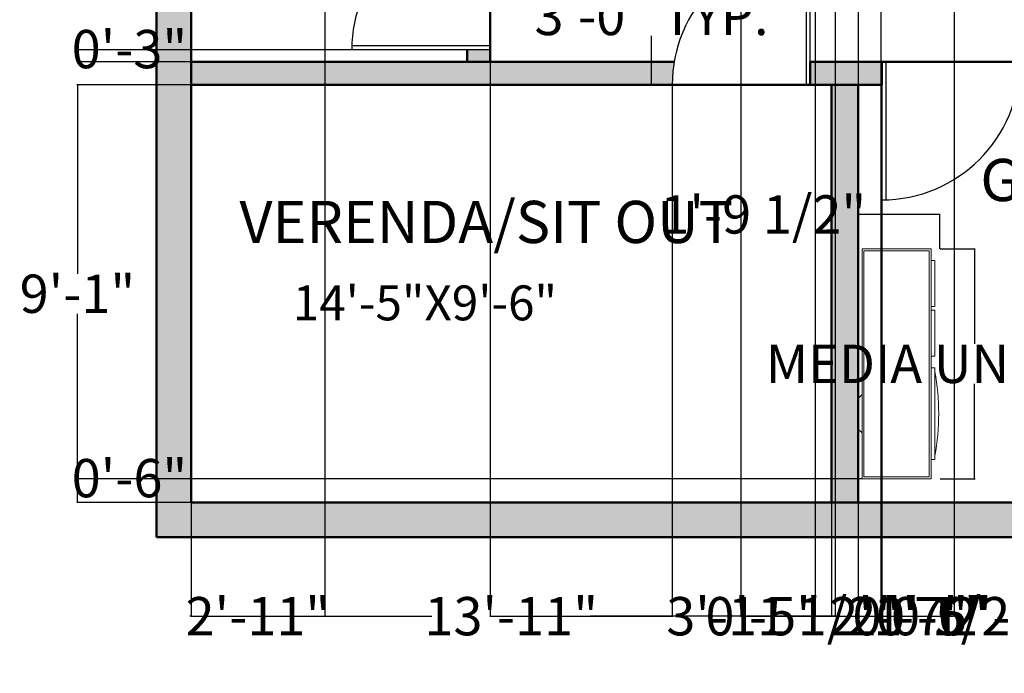
# Model space of a CAD drawing. Units: inches. Extents: x 168 to 640, y -211 to 244.
# Tile 1 of 3: x 179 to 436, y -211 to -40. Entities that reach past the tile are written whole.
import ezdxf

# ---------------------------------------------------------------- set-up
doc = ezdxf.new("R2010")
doc.units = ezdxf.units.IN
doc.header["$MEASUREMENT"] = 0
for name, color, linetype, lineweight in [('A-ANNO-DIMS', 2, 'Continuous', 18), ('A-AREA-IDEN', 7, 'Continuous', 25), ('A-DOOR', 4, 'Continuous', 25), ('A-FURN', 8, 'Continuous', 18), ('A-WALL', 7, 'Continuous', 50)]:
    doc.layers.add(name, color=color, linetype=linetype, lineweight=lineweight)
doc.layers.add('A-WALL-PATT', color=251, linetype='Continuous', lineweight=13, true_color=0x636466)
doc.styles.get("Standard").update_dxf_attribs({"font": 'arial.ttf'})
doc.dimstyles.get("Standard").update_dxf_attribs({"dimtxt": 10, "dimasz": 0.18, "dimexe": 0.18, "dimexo": 0.0625, "dimgap": 0.09, "dimtad": 0, "dimtih": 1, "dimtoh": 1, "dimdec": 0, "dimzin": 0, "dimdsep": 46, "dimlunit": 3, "dimtxsty": 'Standard', "dimcen": 0.09, "dimadec": 0, "dimazin": 0, "dimtfac": 1, "dimtdec": 0, "dimtofl": 0, "dimtmove": 0, "dimatfit": 3, "dimfxl": 1, "dimtolj": 1, "dimtzin": 0, "dimarcsym": 0})

# ---------------------------------------------------------------- blocks, each defined once
blk = doc.blocks.new('Entertainment Center')
for p, q in [((-4, 0), (-5, -1)), ((4, 0), (-4, 0)), ((5, -1), (4, 0)), ((-17, -19), (-17, -1)), ((-17, -1), (43, -1)), ((-16.5, -18.5), (-16.5, -1.5)), ((-16.5, -1.5), (42.5, -1.5)), ((42.5, -1.5), (42.5, -18.5)), ((43, -1), (43, -19)), ((43, -19), (-17, -19)), ((42.5, -18.5), (-16.5, -18.5)), ((-12, -20), (-12, -19)), ((12, -20), (-12, -20)), ((12, -19), (12, -20)), ((15, -20), (15, -19)), ((27, -20), (15, -20)), ((27, -19), (27, -20)), ((28, -20), (28, -19)), ((40, -20), (28, -20)), ((40, -19), (40, -20))]:
    blk.add_line(p, q)
blk.add_arc((0, 40), 61, 259.6111, 280.3889)
blk = doc.blocks.new('DOOR-SWING-36IN')
for p, q in [((0, 36), (0, 0)), ((1, 36), (1, 0))]:
    blk.add_line(p, q)
blk.add_arc((0, 36), 36, 270, 0)
blk = doc.blocks.new('*D12')
at = {"layer": 'A-ANNO-DIMS', "color": 0, "lineweight": -2, "ltscale": 0.25, "transparency": 16777216}
for p, q in [((349.06, -21.2), (343.54, -21.2)), ((343.72, -21.38), (343.72, -34)), ((343.72, -57.02), (343.72, -44.4)), ((349.06, -57.2), (343.54, -57.2))]:
    blk.add_line(p, q, dxfattribs=at)
at = {"layer": 'A-ANNO-DIMS', "color": 0, "ltscale": 0.25, "transparency": 16777216}
for points in [[(343.69, -21.38), (343.75, -21.38), (343.72, -21.2)], [(343.69, -57.02), (343.75, -57.02), (343.72, -57.2)]]:
    blk.add_solid(points, dxfattribs=at)
at = {"layer": 'Defpoints', "color": 0, "ltscale": 0.25, "transparency": 16777216}
for p in [(349.12, -21.2), (343.72, -57.2), (349.12, -57.2)]:
    blk.add_point(p, dxfattribs=at)
at = {"layer": 'A-ANNO-DIMS', "color": 0, "ltscale": 0.25, "transparency": 16777216, "insert": (343.72, -39.2), "char_height": 10, "attachment_point": 5}
blk.add_mtext('\\A1;3\'-0" TYP.', dxfattribs=at)
blk = doc.blocks.new('*D19')
at = {"layer": 'A-ANNO-DIMS', "color": 0, "lineweight": -2, "ltscale": 0.25, "transparency": 16777216}
for p, q in [((419.03, -100), (428.15, -100)), ((427.97, -100.18), (427.97, -124.81)), ((427.97, -159.82), (427.97, -135.2)), ((419.03, -160), (428.15, -160))]:
    blk.add_line(p, q, dxfattribs=at)
at = {"layer": 'A-ANNO-DIMS', "color": 0, "ltscale": 0.25, "transparency": 16777216}
for points in [[(427.94, -100.18), (428, -100.18), (427.97, -100)], [(427.94, -159.82), (428, -159.82), (427.97, -160)]]:
    blk.add_solid(points, dxfattribs=at)
at = {"layer": 'Defpoints', "color": 0, "ltscale": 0.25, "transparency": 16777216}
for p in [(418.97, -100), (427.97, -100), (418.97, -160)]:
    blk.add_point(p, dxfattribs=at)
at = {"layer": 'A-ANNO-DIMS', "color": 0, "ltscale": 0.25, "transparency": 16777216, "insert": (427.97, -130), "char_height": 10, "attachment_point": 5}
blk.add_mtext('\\A1;MEDIA UNIT 5\'-0"', dxfattribs=at)
blk = doc.blocks.new('*D20')
at = {"layer": 'A-ANNO-DIMS', "color": 0, "lineweight": -2, "ltscale": 0.25, "transparency": 16777216}
for p, q in [((397.63, -91), (397.45, -91)), ((397.63, -99.94), (397.63, -90.82)), ((418.79, -91), (397.81, -91)), ((418.97, -99.94), (418.97, -90.82))]:
    blk.add_line(p, q, dxfattribs=at)
at = {"layer": 'A-ANNO-DIMS', "color": 0, "ltscale": 0.25, "transparency": 16777216}
for points in [[(397.81, -90.97), (397.81, -91.03), (397.63, -91)], [(418.79, -90.97), (418.79, -91.03), (418.97, -91)]]:
    blk.add_solid(points, dxfattribs=at)
at = {"layer": 'Defpoints', "color": 0, "ltscale": 0.25, "transparency": 16777216}
for p in [(397.63, -91), (397.63, -100), (418.97, -100)]:
    blk.add_point(p, dxfattribs=at)
at = {"layer": 'A-ANNO-DIMS', "color": 0, "ltscale": 0.25, "transparency": 16777216, "insert": (372.89, -91), "char_height": 10, "attachment_point": 5}
blk.add_mtext('\\A1;1\'-9 1/2"', dxfattribs=at)
blk = doc.blocks.new('*D28')
at = {"layer": 'A-ANNO-DIMS', "color": 0, "lineweight": -2, "ltscale": 0.25, "transparency": 16777216}
for p, q in [((390.63, -166.26), (390.63, -196.03)), ((397.63, -166.26), (397.63, -196.03)), ((390.81, -195.85), (397.45, -195.85)), ((397.63, -195.85), (397.81, -195.85))]:
    blk.add_line(p, q, dxfattribs=at)
at = {"layer": 'A-ANNO-DIMS', "color": 0, "ltscale": 0.25, "transparency": 16777216}
for points in [[(390.81, -195.82), (390.81, -195.88), (390.63, -195.85)], [(397.45, -195.82), (397.45, -195.88), (397.63, -195.85)]]:
    blk.add_solid(points, dxfattribs=at)
at = {"layer": 'Defpoints', "color": 0, "ltscale": 0.25, "transparency": 16777216}
for p in [(390.63, -166.2), (397.63, -166.2), (397.63, -195.85)]:
    blk.add_point(p, dxfattribs=at)
at = {"layer": 'A-ANNO-DIMS', "color": 0, "ltscale": 0.25, "transparency": 16777216, "insert": (411.2, -195.85), "char_height": 10, "attachment_point": 5}
blk.add_mtext('\\A1;0\'-7"', dxfattribs=at)
blk = doc.blocks.new('*D29')
at = {"layer": 'A-ANNO-DIMS', "color": 0, "lineweight": -2, "ltscale": 0.25, "transparency": 16777216}
for p, q in [((223.63, -166.26), (223.63, -196.03)), ((390.63, -166.26), (390.63, -196.03)), ((223.81, -195.85), (286.45, -195.85)), ((390.45, -195.85), (327.81, -195.85))]:
    blk.add_line(p, q, dxfattribs=at)
at = {"layer": 'A-ANNO-DIMS', "color": 0, "ltscale": 0.25, "transparency": 16777216}
for points in [[(223.81, -195.82), (223.81, -195.88), (223.63, -195.85)], [(390.45, -195.82), (390.45, -195.88), (390.63, -195.85)]]:
    blk.add_solid(points, dxfattribs=at)
at = {"layer": 'Defpoints', "color": 0, "ltscale": 0.25, "transparency": 16777216}
for p in [(223.63, -166.2), (390.63, -166.2), (390.63, -195.85)]:
    blk.add_point(p, dxfattribs=at)
at = {"layer": 'A-ANNO-DIMS', "color": 0, "ltscale": 0.25, "transparency": 16777216, "insert": (307.13, -195.85), "char_height": 10, "attachment_point": 5}
blk.add_mtext('\\A1;13\'-11"', dxfattribs=at)
blk = doc.blocks.new('*D30')
at = {"layer": 'A-ANNO-DIMS', "color": 0, "lineweight": -2, "ltscale": 0.25, "transparency": 16777216}
for p, q in [((223.57, -57.2), (193.8, -57.2)), ((193.98, -57.38), (193.98, -106.5)), ((193.98, -166.02), (193.98, -116.9)), ((223.57, -166.2), (193.8, -166.2))]:
    blk.add_line(p, q, dxfattribs=at)
at = {"layer": 'A-ANNO-DIMS', "color": 0, "ltscale": 0.25, "transparency": 16777216}
for points in [[(193.95, -57.38), (194.01, -57.38), (193.98, -57.2)], [(193.95, -166.02), (194.01, -166.02), (193.98, -166.2)]]:
    blk.add_solid(points, dxfattribs=at)
at = {"layer": 'Defpoints', "color": 0, "ltscale": 0.25, "transparency": 16777216}
for p in [(193.98, -57.2), (223.63, -57.2), (223.63, -166.2)]:
    blk.add_point(p, dxfattribs=at)
at = {"layer": 'A-ANNO-DIMS', "color": 0, "ltscale": 0.25, "transparency": 16777216, "insert": (193.98, -111.7), "char_height": 10, "attachment_point": 5}
blk.add_mtext('\\A1;9\'-1"', dxfattribs=at)
blk = doc.blocks.new('*D35')
at = {"layer": 'A-ANNO-DIMS', "color": 0, "lineweight": -2, "ltscale": 0.25, "transparency": 16777216}
for p, q in [((386.42, 73.74), (386.42, -196.03)), ((403.56, 73.74), (403.56, -196.03)), ((386.6, -195.85), (403.38, -195.85)), ((403.56, -195.85), (403.74, -195.85))]:
    blk.add_line(p, q, dxfattribs=at)
at = {"layer": 'A-ANNO-DIMS', "color": 0, "ltscale": 0.25, "transparency": 16777216}
for points in [[(386.6, -195.82), (386.6, -195.88), (386.42, -195.85)], [(403.38, -195.82), (403.38, -195.88), (403.56, -195.85)]]:
    blk.add_solid(points, dxfattribs=at)
at = {"layer": 'Defpoints', "color": 0, "ltscale": 0.25, "transparency": 16777216}
for p in [(386.42, 73.8), (403.56, 73.8), (403.56, -195.85)]:
    blk.add_point(p, dxfattribs=at)
at = {"layer": 'A-ANNO-DIMS', "color": 0, "ltscale": 0.25, "transparency": 16777216, "insert": (416.65, -195.85), "char_height": 10, "attachment_point": 5}
blk.add_mtext('\\A1;1\'-5"', dxfattribs=at)
blk = doc.blocks.new('*D36')
at = {"layer": 'A-ANNO-DIMS', "color": 0, "lineweight": -2, "ltscale": 0.25, "transparency": 16777216}
for p, q in [((386.42, 79.74), (386.42, -196.03)), ((391.63, 79.74), (391.63, -196.03)), ((386.42, -195.85), (386.24, -195.85)), ((391.45, -195.85), (386.6, -195.85))]:
    blk.add_line(p, q, dxfattribs=at)
at = {"layer": 'A-ANNO-DIMS', "color": 0, "ltscale": 0.25, "transparency": 16777216}
for points in [[(386.6, -195.82), (386.6, -195.88), (386.42, -195.85)], [(391.45, -195.82), (391.45, -195.88), (391.63, -195.85)]]:
    blk.add_solid(points, dxfattribs=at)
at = {"layer": 'Defpoints', "color": 0, "ltscale": 0.25, "transparency": 16777216}
for p in [(386.42, 79.8), (391.63, 79.8), (386.42, -195.85)]:
    blk.add_point(p, dxfattribs=at)
at = {"layer": 'A-ANNO-DIMS', "color": 0, "ltscale": 0.25, "transparency": 16777216, "insert": (372.86, -195.85), "char_height": 10, "attachment_point": 5}
blk.add_mtext('\\A1;0\'-5"', dxfattribs=at)
blk = doc.blocks.new('*D37')
at = {"layer": 'A-ANNO-DIMS', "color": 0, "lineweight": -2, "ltscale": 0.25, "transparency": 16777216}
for p, q in [((301.63, -51.26), (301.63, -196.03)), ((349.12, -57.26), (349.12, -196.03)), ((301.81, -195.85), (348.94, -195.85)), ((349.12, -195.85), (349.3, -195.85))]:
    blk.add_line(p, q, dxfattribs=at)
at = {"layer": 'A-ANNO-DIMS', "color": 0, "ltscale": 0.25, "transparency": 16777216}
for points in [[(301.81, -195.82), (301.81, -195.88), (301.63, -195.85)], [(348.94, -195.82), (348.94, -195.88), (349.12, -195.85)]]:
    blk.add_solid(points, dxfattribs=at)
at = {"layer": 'Defpoints', "color": 0, "ltscale": 0.25, "transparency": 16777216}
for p in [(301.63, -51.2), (349.12, -57.2), (349.12, -195.85)]:
    blk.add_point(p, dxfattribs=at)
at = {"layer": 'A-ANNO-DIMS', "color": 0, "ltscale": 0.25, "transparency": 16777216, "insert": (378.21, -195.85), "char_height": 10, "attachment_point": 5}
blk.add_mtext('\\A1;3\'-11 1/2"', dxfattribs=at)
blk = doc.blocks.new('*D38')
at = {"layer": 'A-ANNO-DIMS', "color": 0, "lineweight": -2, "ltscale": 0.25, "transparency": 16777216}
for p, q in [((397.63, -57.26), (397.63, -196.03)), ((403.8, -57.26), (403.8, -196.03)), ((397.81, -195.85), (403.62, -195.85)), ((403.8, -195.85), (403.98, -195.85))]:
    blk.add_line(p, q, dxfattribs=at)
at = {"layer": 'A-ANNO-DIMS', "color": 0, "ltscale": 0.25, "transparency": 16777216}
for points in [[(397.81, -195.82), (397.81, -195.88), (397.63, -195.85)], [(403.62, -195.82), (403.62, -195.88), (403.8, -195.85)]]:
    blk.add_solid(points, dxfattribs=at)
at = {"layer": 'Defpoints', "color": 0, "ltscale": 0.25, "transparency": 16777216}
for p in [(397.63, -57.2), (403.8, -57.2), (403.8, -195.85)]:
    blk.add_point(p, dxfattribs=at)
at = {"layer": 'A-ANNO-DIMS', "color": 0, "ltscale": 0.25, "transparency": 16777216, "insert": (417.37, -195.85), "char_height": 10, "attachment_point": 5}
blk.add_mtext('\\A1;0\'-6"', dxfattribs=at)
blk = doc.blocks.new('*D39')
at = {"layer": 'A-ANNO-DIMS', "color": 0, "lineweight": -2, "ltscale": 0.25, "transparency": 16777216}
for p, q in [((295.57, -48.03), (193.8, -48.03)), ((193.98, -48.03), (193.98, -47.85)), ((193.98, -47.85), (194.16, -47.85)), ((193.98, -51.02), (193.98, -48.21)), ((295.57, -51.2), (193.8, -51.2))]:
    blk.add_line(p, q, dxfattribs=at)
at = {"layer": 'A-ANNO-DIMS', "color": 0, "ltscale": 0.25, "transparency": 16777216}
for points in [[(193.95, -48.21), (194.01, -48.21), (193.98, -48.03)], [(193.95, -51.02), (194.01, -51.02), (193.98, -51.2)]]:
    blk.add_solid(points, dxfattribs=at)
at = {"layer": 'Defpoints', "color": 0, "ltscale": 0.25, "transparency": 16777216}
for p in [(193.98, -48.03), (295.63, -48.03), (295.63, -51.2)]:
    blk.add_point(p, dxfattribs=at)
at = {"layer": 'A-ANNO-DIMS', "color": 0, "ltscale": 0.25, "transparency": 16777216, "insert": (207.55, -47.85), "char_height": 10, "attachment_point": 5}
blk.add_mtext('\\A1;0\'-3"', dxfattribs=at)
blk = doc.blocks.new('*D45')
at = {"layer": 'A-ANNO-DIMS', "color": 0, "lineweight": -2, "ltscale": 0.25, "transparency": 16777216}
for p, q in [((223.63, -20.98), (223.63, -196.03)), ((258.47, -20.98), (258.47, -196.03)), ((223.45, -195.85), (223.27, -195.85)), ((258.65, -195.85), (258.83, -195.85))]:
    blk.add_line(p, q, dxfattribs=at)
at = {"layer": 'A-ANNO-DIMS', "color": 0, "ltscale": 0.25, "transparency": 16777216}
for points in [[(223.45, -195.82), (223.45, -195.88), (223.63, -195.85)], [(258.65, -195.82), (258.65, -195.88), (258.47, -195.85)]]:
    blk.add_solid(points, dxfattribs=at)
at = {"layer": 'Defpoints', "color": 0, "ltscale": 0.25, "transparency": 16777216}
for p in [(223.63, -20.92), (258.47, -20.92), (258.47, -195.85)]:
    blk.add_point(p, dxfattribs=at)
at = {"layer": 'A-ANNO-DIMS', "color": 0, "ltscale": 0.25, "transparency": 16777216, "insert": (241.05, -195.85), "char_height": 10, "attachment_point": 5}
blk.add_mtext('\\A1;2\'-11"', dxfattribs=at)
blk = doc.blocks.new('*D53')
at = {"layer": 'A-ANNO-DIMS', "color": 0, "lineweight": -2, "ltscale": 0.25, "transparency": 16777216}
for p, q in [((367.04, 124.86), (367.04, -196.03)), ((391.63, 124.86), (391.63, -196.03)), ((367.22, -195.85), (391.45, -195.85)), ((391.63, -195.85), (391.81, -195.85))]:
    blk.add_line(p, q, dxfattribs=at)
at = {"layer": 'A-ANNO-DIMS', "color": 0, "ltscale": 0.25, "transparency": 16777216}
for points in [[(367.22, -195.82), (367.22, -195.88), (367.04, -195.85)], [(391.45, -195.82), (391.45, -195.88), (391.63, -195.85)]]:
    blk.add_solid(points, dxfattribs=at)
at = {"layer": 'Defpoints', "color": 0, "ltscale": 0.25, "transparency": 16777216}
for p in [(367.04, 124.92), (391.63, 124.92), (391.63, -195.85)]:
    blk.add_point(p, dxfattribs=at)
at = {"layer": 'A-ANNO-DIMS', "color": 0, "ltscale": 0.25, "transparency": 16777216, "insert": (416.93, -195.85), "char_height": 10, "attachment_point": 5}
blk.add_mtext('\\A1;2\'-0 1/2"', dxfattribs=at)
blk = doc.blocks.new('*D55')
at = {"layer": 'A-ANNO-DIMS', "color": 0, "lineweight": -2, "ltscale": 0.25, "transparency": 16777216}
for p, q in [((397.63, 124.86), (397.63, -196.03)), ((422.63, 124.86), (422.63, -196.03)), ((397.81, -195.85), (422.45, -195.85)), ((422.63, -195.85), (422.81, -195.85))]:
    blk.add_line(p, q, dxfattribs=at)
at = {"layer": 'A-ANNO-DIMS', "color": 0, "ltscale": 0.25, "transparency": 16777216}
for points in [[(397.81, -195.82), (397.81, -195.88), (397.63, -195.85)], [(422.45, -195.82), (422.45, -195.88), (422.63, -195.85)]]:
    blk.add_solid(points, dxfattribs=at)
at = {"layer": 'Defpoints', "color": 0, "ltscale": 0.25, "transparency": 16777216}
for p in [(397.63, 124.92), (422.63, 124.92), (422.63, -195.85)]:
    blk.add_point(p, dxfattribs=at)
at = {"layer": 'A-ANNO-DIMS', "color": 0, "ltscale": 0.25, "transparency": 16777216, "insert": (436.28, -195.85), "char_height": 10, "attachment_point": 5}
blk.add_mtext('\\A1;2\'-1"', dxfattribs=at)
blk = doc.blocks.new('*D59')
at = {"layer": 'A-ANNO-DIMS', "color": 0, "lineweight": -2, "ltscale": 0.25, "transparency": 16777216}
for p, q in [((398.57, -160), (193.8, -160)), ((193.98, -160), (193.98, -159.82)), ((193.98, -159.82), (194.16, -159.82)), ((193.98, -166.02), (193.98, -160.18)), ((397.57, -166.2), (193.8, -166.2))]:
    blk.add_line(p, q, dxfattribs=at)
at = {"layer": 'A-ANNO-DIMS', "color": 0, "ltscale": 0.25, "transparency": 16777216}
for points in [[(193.95, -160.18), (194.01, -160.18), (193.98, -160)], [(193.95, -166.02), (194.01, -166.02), (193.98, -166.2)]]:
    blk.add_solid(points, dxfattribs=at)
at = {"layer": 'Defpoints', "color": 0, "ltscale": 0.25, "transparency": 16777216}
for p in [(193.98, -160), (398.63, -160), (397.63, -166.2)]:
    blk.add_point(p, dxfattribs=at)
at = {"layer": 'A-ANNO-DIMS', "color": 0, "ltscale": 0.25, "transparency": 16777216, "insert": (207.55, -159.82), "char_height": 10, "attachment_point": 5}
blk.add_mtext('\\A1;0\'-6"', dxfattribs=at)

msp = doc.modelspace()

# ---------------------------------------------------------------- hatches: boundary and pattern name
at = {"layer": 'A-WALL-PATT', "ltscale": 0.25}
h = msp.add_hatch(color=256, dxfattribs=at)
h.dxf.hatch_style = 1
h.paths.add_polyline_path([(223.63, 11.3), (214.63, 11.3), (214.63, -175.2), (574.63, -175.2), (574.63, -137.43), (565.63, -137.43), (565.63, -157.06), (565.63, -166.2), (223.63, -166.2)])
h.paths.add_polyline_path([(349.62, -51.2), (301.63, -51.2), (223.63, -51.2), (223.63, -57.2), (301.63, -57.2), (349.12, -57.2, -0.041886)], flags=17)
h.paths.add_polyline_path([(301.63, -48.03), (295.63, -48.03), (295.63, -51.2), (301.63, -51.2)], flags=17)
h.paths.add_polyline_path([(403.8, -51.2), (385.12, -51.2), (385.12, -57.2), (403.8, -57.2)], flags=17)
h.paths.add_polyline_path([(397.63, -57.2), (390.63, -57.2), (390.63, -166.2), (397.63, -166.2)], flags=17)
h.paths.add_polyline_path([(301.63, 73.8), (295.63, 73.8), (295.63, -12.53, -0.041886), (301.63, -12.03)])
h.paths.add_polyline_path([(223.63, 122.57), (214.63, 122.57), (214.63, 47.3), (223.63, 47.3), (223.63, 73.8)])
h.paths.add_polyline_path([(350.92, 79.8), (223.63, 79.8), (223.63, 73.8), (350.42, 73.8, -0.041886)])
h.paths.add_polyline_path([(574.63, 208.8), (214.63, 208.8), (214.63, 158.57), (223.63, 158.57), (223.63, 199.8), (565.63, 199.8), (565.63, 158.57), (574.63, 158.57)])
h.paths.add_polyline_path([(397.63, 199.8), (391.63, 199.8), (391.63, 79.8), (386.42, 79.8), (386.42, 73.8), (391.63, 73.8), (403.56, 73.8), (403.56, 79.8), (397.63, 79.8)])
h.paths.add_polyline_path([(565.63, 79.8), (439.06, 79.8, -0.041886), (439.56, 73.8), (565.63, 73.8)])
h.paths.add_polyline_path([(574.63, 122.57), (565.63, 122.57), (565.63, 79.8), (565.63, 52.8), (574.63, 52.8)])
h.paths.add_polyline_path([(574.63, 16.8), (565.63, 16.8), (565.63, -15.33), (574.63, -15.33)])
h.paths.add_polyline_path([(574.63, -39.29), (570.13, -39.29), (565.63, -39.29), (565.63, -51.2), (565.63, -101.43), (574.63, -101.43)], flags=17)
h.paths.add_polyline_path([(565.63, -51.2), (439.8, -51.2, -0.041886), (439.3, -57.2), (565.63, -57.2)], flags=17)

# ---------------------------------------------------------------- linework, layer by layer
at = {"layer": 'A-DOOR'}
msp.add_line((301.63, -47.03), (301.63, -48.03), dxfattribs=at)
at = {"layer": 'A-WALL'}
for p, q in [((214.63, 208.8), (214.63, -175.2)), ((223.63, 199.8), (223.63, -166.2)), ((223.63, 73.8), (223.63, -51.2)), ((301.63, -51.2), (301.63, 73.8)), ((295.63, -51.2), (295.63, -48.03)), ((223.63, -51.2), (301.63, -51.2)), ((349.62, -51.2), (301.63, -51.2)), ((565.63, -51.2), (385.12, -51.2)), ((385.12, -57.2), (385.12, -51.2)), ((403.8, -57.2), (403.8, -51.2)), ((223.63, -57.2), (301.63, -57.2)), ((403.8, -57.2), (301.63, -57.2)), ((390.63, -57.2), (390.63, -166.2)), ((397.63, -57.2), (397.63, -166.2)), ((223.63, -166.2), (565.63, -166.2)), ((214.63, -175.2), (574.63, -175.2))]:
    msp.add_line(p, q, dxfattribs=at)

# ---------------------------------------------------------------- block references
at = {"layer": 'A-DOOR', "extrusion": (0, 0, -1), "zscale": -1, "rotation": 90.00000000000007}
msp.add_blockref('DOOR-SWING-36IN', (-265.63, -48.03), dxfattribs=at)
at = {"layer": 'A-DOOR', "rotation": 180}
msp.add_blockref('DOOR-SWING-36IN', (385.12, -21.2), dxfattribs=at)
at = {"layer": 'A-DOOR'}
msp.add_blockref('DOOR-SWING-36IN', (403.8, -87.2), dxfattribs=at)
at = {"layer": 'A-FURN', "ltscale": 0.25, "rotation": 90}
msp.add_blockref('Entertainment Center', (397.63, -143), dxfattribs=at)

# ---------------------------------------------------------------- texts
at = {"layer": 'A-AREA-IDEN', "ltscale": 0.25}
for s, height, p in [('GUEST/DRAWING', 11.0125, (429.5, -87.52)), ('VERENDA/SIT OUT  ', 11.0125, (236.23, -98.47)), ('14\'-5"X9\'-6"', 9.1115, (250.15, -118.64))]:
    msp.add_text(s, height=height, dxfattribs=at).set_placement(p)

# ---------------------------------------------------------------- dimensions: what is measured, and where the dimension line sits
at = {"layer": 'A-ANNO-DIMS', "ltscale": 0.25}
for base, p1, p2, picture, middle in [((391.63, -195.85), (367.04, 124.92), (391.63, 124.92), '*D53', (416.93, -195.85)), ((422.63, -195.85), (397.63, 124.92), (422.63, 124.92), '*D55', (436.28, -195.85)), ((386.42, -195.85), (391.63, 79.8), (386.42, 79.8), '*D36', (372.86, -195.85)), ((403.56, -195.85), (386.42, 73.8), (403.56, 73.8), '*D35', (416.65, -195.85)), ((258.47, -195.85), (223.63, -20.92), (258.47, -20.92), '*D45', (241.05, -195.85)), ((349.12, -195.85), (301.63, -51.2), (349.12, -57.2), '*D37', (378.21, -195.85)), ((403.8, -195.85), (397.63, -57.2), (403.8, -57.2), '*D38', (417.37, -195.85)), ((390.63, -195.85), (223.63, -166.2), (390.63, -166.2), '*D29', (307.13, -195.85)), ((397.63, -195.85), (390.63, -166.2), (397.63, -166.2), '*D28', (411.2, -195.85))]:
    dim = msp.add_linear_dim(base=base, p1=p1, p2=p2, dimstyle='Standard', override={"dimdec": 1, "dimlfac": 1, "dimrnd": 0, "dimzin": 1, "dimdsep": 46, "dimlunit": 4, "dimfrac": 2}, dxfattribs=at)
    dim.commit()
    dim.dimension.update_dxf_attribs({"geometry": picture, "text_midpoint": middle})
for base, p1, p2, angle, text, picture, middle in [((343.72, -57.2), (349.12, -21.2), (349.12, -57.2), 270, '<> TYP.', '*D12', (343.72, -39.2)), ((427.97, -100), (418.97, -160), (418.97, -100), 90, 'MEDIA UNIT <>', '*D19', (427.97, -130))]:
    dim = msp.add_linear_dim(base=base, p1=p1, p2=p2, angle=angle, text=text, dimstyle='Standard', override={"dimdec": 1, "dimlfac": 1, "dimrnd": 0, "dimzin": 1, "dimdsep": 46, "dimlunit": 4, "dimfrac": 2}, dxfattribs=at)
    dim.commit()
    dim.dimension.update_dxf_attribs({"geometry": picture, "text_midpoint": middle})
for base, p1, p2, angle, picture, middle in [((193.98, -48.03), (295.63, -51.2), (295.63, -48.03), 90, '*D39', (207.55, -47.85)), ((193.98, -57.2), (223.63, -166.2), (223.63, -57.2), 90, '*D30', (193.98, -111.7)), ((397.63, -91), (418.97, -100), (397.63, -100), 180, '*D20', (372.89, -91)), ((193.98, -160), (397.63, -166.2), (398.63, -160), 90, '*D59', (207.55, -159.82))]:
    dim = msp.add_linear_dim(base=base, p1=p1, p2=p2, angle=angle, dimstyle='Standard', override={"dimdec": 1, "dimlfac": 1, "dimrnd": 0, "dimzin": 1, "dimdsep": 46, "dimlunit": 4, "dimfrac": 2}, dxfattribs=at)
    dim.commit()
    dim.dimension.update_dxf_attribs({"geometry": picture, "text_midpoint": middle})

doc.saveas('drawing.dxf')
